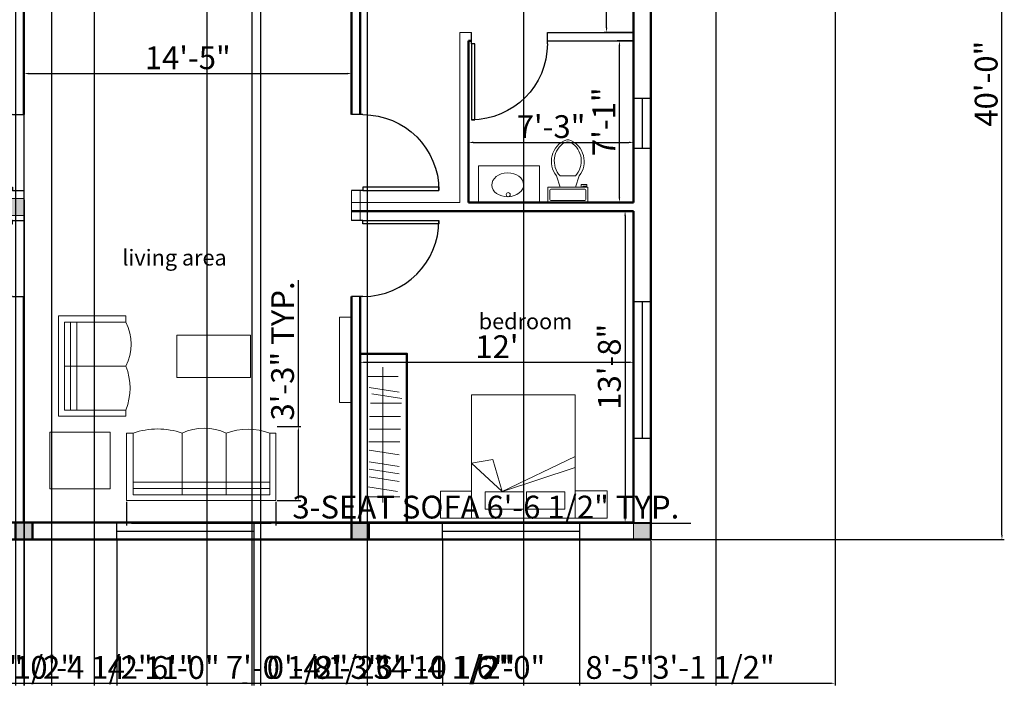
# Model space of a CAD drawing. Units: inches. Extents: x 1367 to 2309, y 1406 to 3826.
# Tile 5 of 9: x 1781 to 2300, y 2247 to 2608. Entities that reach past the tile are written whole.
import ezdxf

# ---------------------------------------------------------------- set-up
doc = ezdxf.new("R2010")
doc.units = ezdxf.units.IN
for name, color, linetype, lineweight in [('A-ANNO-DIMS', 2, 'Continuous', 18), ('A-AREA-IDEN', 3, 'Continuous', 18), ('A-DOOR', 4, 'Continuous', 25), ('A-FLOR-FIXT', 8, 'Continuous', 18), ('A-FURN', 8, 'Continuous', 18), ('A-GLAZ', 4, 'Continuous', 25), ('A-WALL', 7, 'Continuous', 50), ('A-WALL-PATT', 8, 'Continuous', 18)]:
    doc.layers.add(name, color=color, linetype=linetype, lineweight=lineweight)
doc.styles.get("Standard").update_dxf_attribs({"font": 'arial.ttf'})
doc.dimstyles.new('ISO-25', dxfattribs={"dimtxt": 12, "dimasz": 2.5, "dimexe": 1.25, "dimexo": 0.625, "dimtad": 1, "dimdec": 0, "dimlunit": 4, "dimtxsty": 'Standard', "dimcen": 2.5, "dimadec": 0, "dimazin": 0, "dimtfac": 1, "dimtdec": 0, "dimtmove": 0, "dimatfit": 3, "dimfxl": 1, "dimarcsym": 0})

# ---------------------------------------------------------------- blocks, each defined once
blk = doc.blocks.new('*U2')
for p, q in [((0, 0), (0, -6)), ((40, 0), (40, -6))]:
    blk.add_line(p, q)
blk.add_lwpolyline([(0, 0), (0, 40), (1.75, 40), (1.75, 0)], close=True)
blk.add_arc((0, 0), 40, 0, 90)
blk = doc.blocks.new('*U4')
for p, q in [((9.5, -6), (9.5, -2)), ((-10, -8.5), (-8, -8.5)), ((-10, -9.5), (-10, -8.5)), ((-7, -9.5), (-10, -9.5)), ((-8, -8.5), (-8, -8)), ((-7, -8), (-7, -9.5)), ((-4, -8), (-6, -14)), ((4, -8), (6, -14)), ((4, -14), (-4, -14))]:
    blk.add_line(p, q)
blk.add_lwpolyline([(10.5, -8), (10.5, 0), (-10.5, 0), (-10.5, -8)], close=True)
for points in [[(-9.5, -2), (-9.5, -6)], [(8.5, -1), (-8.5, -1)], [(-8.5, -7), (8.5, -7)]]:
    blk.add_lwpolyline(points)
for centre, radius, start, end in [((-8.62, -1.88), 0.884, 81.8699, 188.1301), ((8.62, -1.88), 0.884, 351.8699, 98.1301), ((-8.62, -6.12), 0.884, 171.8699, 278.1301), ((8.62, -6.12), 0.884, 261.8699, 8.1301), ((3.52, -21.58), 12.17, 141.4691, 247.9714), ((4.2, -21.82), 11.33, 136.3677, 238.9468), ((-3.52, -21.58), 12.17, 292.0284, 38.5307), ((-4.2, -21.82), 11.33, 301.053, 43.6321), ((0, -27.88), 4, 245.7318, 294.2682), ((0, -29), 4, 254.8605, 285.1395)]:
    blk.add_arc(centre, radius, start, end)
blk = doc.blocks.new('*D16')
at = {"layer": 'A-ANNO-DIMS', "color": 0, "lineweight": -2, "transparency": 16777216}
for p, q in [((2103.75, 2805.17), (2088.85, 2805.17)), ((2090.1, 2603.67), (2090.1, 2802.67)), ((2103.75, 2601.17), (2088.85, 2601.17))]:
    blk.add_line(p, q, dxfattribs=at)
at = {"layer": 'A-ANNO-DIMS', "color": 0, "lineweight": 100, "transparency": 16777216}
for points in [[(2089.68, 2802.67), (2090.51, 2802.67), (2090.1, 2805.17)], [(2089.68, 2603.67), (2090.51, 2603.67), (2090.1, 2601.17)]]:
    blk.add_solid(points, dxfattribs=at)
at = {"layer": 'Defpoints', "color": 0, "lineweight": 100, "transparency": 16777216}
for p in [(2090.1, 2805.17), (2104.37, 2805.17), (2104.37, 2601.17)]:
    blk.add_point(p, dxfattribs=at)
at = {"layer": 'A-ANNO-DIMS', "color": 0, "transparency": 16777216, "insert": (2083.45, 2703.17), "char_height": 12, "attachment_point": 5, "rotation": 90}
blk.add_mtext("17'", dxfattribs=at)
blk = doc.blocks.new('*D17')
at = {"layer": 'A-ANNO-DIMS', "color": 0, "lineweight": -2, "transparency": 16777216}
for p, q in [((2103.75, 2596.67), (2095.64, 2596.67)), ((2096.89, 2514.16), (2096.89, 2594.17)), ((2103.75, 2511.66), (2095.64, 2511.66))]:
    blk.add_line(p, q, dxfattribs=at)
at = {"layer": 'A-ANNO-DIMS', "color": 0, "lineweight": 100, "transparency": 16777216}
for points in [[(2096.47, 2594.17), (2097.3, 2594.17), (2096.89, 2596.67)], [(2096.47, 2514.16), (2097.3, 2514.16), (2096.89, 2511.66)]]:
    blk.add_solid(points, dxfattribs=at)
at = {"layer": 'Defpoints', "color": 0, "lineweight": 100, "transparency": 16777216}
for p in [(2096.89, 2596.67), (2104.37, 2596.67), (2104.37, 2511.66)]:
    blk.add_point(p, dxfattribs=at)
at = {"layer": 'A-ANNO-DIMS', "color": 0, "transparency": 16777216, "insert": (2090.24, 2554.16), "char_height": 12, "attachment_point": 5, "rotation": 90}
blk.add_mtext('7\'-1"', dxfattribs=at)
blk = doc.blocks.new('*D18')
at = {"layer": 'A-ANNO-DIMS', "color": 0, "lineweight": -2, "transparency": 16777216}
for p, q in [((2017.4, 2512.28), (2017.4, 2544.52)), ((2019.9, 2543.27), (2101.87, 2543.27)), ((2104.37, 2512.28), (2104.37, 2544.52))]:
    blk.add_line(p, q, dxfattribs=at)
at = {"layer": 'A-ANNO-DIMS', "color": 0, "lineweight": 100, "transparency": 16777216}
for points in [[(2019.9, 2543.69), (2019.9, 2542.86), (2017.4, 2543.27)], [(2101.87, 2543.69), (2101.87, 2542.86), (2104.37, 2543.27)]]:
    blk.add_solid(points, dxfattribs=at)
at = {"layer": 'Defpoints', "color": 0, "lineweight": 100, "transparency": 16777216}
for p in [(2104.37, 2543.27), (2017.4, 2511.66), (2104.37, 2511.66)]:
    blk.add_point(p, dxfattribs=at)
at = {"layer": 'A-ANNO-DIMS', "color": 0, "transparency": 16777216, "insert": (2060.89, 2550.03), "char_height": 12, "attachment_point": 5}
blk.add_mtext('7\'-3"', dxfattribs=at)
blk = doc.blocks.new('*D19')
at = {"layer": 'A-ANNO-DIMS', "color": 0, "lineweight": -2, "transparency": 16777216}
for p, q in [((1960.37, 2343.79), (1960.37, 2428.77)), ((1962.87, 2427.52), (2101.87, 2427.52)), ((2104.37, 2343.79), (2104.37, 2428.77))]:
    blk.add_line(p, q, dxfattribs=at)
at = {"layer": 'A-ANNO-DIMS', "color": 0, "lineweight": 100, "transparency": 16777216}
for points in [[(1962.87, 2427.93), (1962.87, 2427.1), (1960.37, 2427.52)], [(2101.87, 2427.93), (2101.87, 2427.1), (2104.37, 2427.52)]]:
    blk.add_solid(points, dxfattribs=at)
at = {"layer": 'Defpoints', "color": 0, "lineweight": 100, "transparency": 16777216}
for p in [(2104.37, 2427.52), (1960.37, 2343.17), (2104.37, 2343.17)]:
    blk.add_point(p, dxfattribs=at)
at = {"layer": 'A-ANNO-DIMS', "color": 0, "transparency": 16777216, "insert": (2032.37, 2434.17), "char_height": 12, "attachment_point": 5}
blk.add_mtext("12'", dxfattribs=at)
blk = doc.blocks.new('*D20')
at = {"layer": 'A-ANNO-DIMS', "color": 0, "lineweight": -2, "transparency": 16777216}
for p, q in [((2103.75, 2507.16), (2098.62, 2507.16)), ((2099.87, 2504.66), (2099.87, 2345.67)), ((2103.75, 2343.17), (2098.62, 2343.17))]:
    blk.add_line(p, q, dxfattribs=at)
at = {"layer": 'A-ANNO-DIMS', "color": 0, "lineweight": 100, "transparency": 16777216}
for points in [[(2099.46, 2504.66), (2100.29, 2504.66), (2099.87, 2507.16)], [(2099.46, 2345.67), (2100.29, 2345.67), (2099.87, 2343.17)]]:
    blk.add_solid(points, dxfattribs=at)
at = {"layer": 'Defpoints', "color": 0, "lineweight": 100, "transparency": 16777216}
for p in [(2104.37, 2507.16), (2099.87, 2343.17), (2104.37, 2343.17)]:
    blk.add_point(p, dxfattribs=at)
at = {"layer": 'A-ANNO-DIMS', "color": 0, "transparency": 16777216, "insert": (2093.12, 2425.16), "char_height": 12, "attachment_point": 5, "rotation": 90}
blk.add_mtext('13\'-8"', dxfattribs=at)
blk = doc.blocks.new('*D37')
at = {"layer": 'A-ANNO-DIMS', "color": 0, "lineweight": -2, "transparency": 16777216}
for p, q in [((1783.37, 2558.52), (1783.37, 2580.77)), ((1785.87, 2579.52), (1953.37, 2579.52)), ((1955.87, 2558.52), (1955.87, 2580.77))]:
    blk.add_line(p, q, dxfattribs=at)
at = {"layer": 'A-ANNO-DIMS', "color": 0, "lineweight": 100, "transparency": 16777216}
for points in [[(1785.87, 2579.94), (1785.87, 2579.1), (1783.37, 2579.52)], [(1953.37, 2579.94), (1953.37, 2579.1), (1955.87, 2579.52)]]:
    blk.add_solid(points, dxfattribs=at)
at = {"layer": 'Defpoints', "color": 0, "lineweight": 100, "transparency": 16777216}
for p in [(1955.87, 2579.52), (1783.37, 2557.89), (1955.87, 2557.89)]:
    blk.add_point(p, dxfattribs=at)
at = {"layer": 'A-ANNO-DIMS', "color": 0, "transparency": 16777216, "insert": (1869.62, 2586.27), "char_height": 12, "attachment_point": 5}
blk.add_mtext('14\'-5"', dxfattribs=at)
blk = doc.blocks.new('SOFA-3')
for p, q in [((3.39, 35.52), (0, 35.52)), ((0, 35.52), (0, 0)), ((29.28, 35.52), (29.28, 3.13)), ((52.37, 35.52), (52.37, 3.13)), ((75.45, 35.52), (78.61, 35.52)), ((78.61, 0), (78.61, 35.52)), ((0, 0), (78.61, 0))]:
    blk.add_line(p, q)
blk.add_lwpolyline([(3.39, 35.52), (3.39, 3.13), (75.45, 3.13), (75.45, 35.52)])
for centre, radius, start, end in [((16.33, -1.36), 39.09, 70.661, 109.339), ((40.82, 12.11), 26.1, 63.7496, 116.2504), ((63.91, 5.49), 32.17, 68.9718, 111.0282)]:
    blk.add_arc(centre, radius, start, end)
blk = doc.blocks.new('ARMCHAIR')
for p, q in [((0, 52.73), (0, 0)), ((35.52, 52.73), (0, 52.73)), ((35.52, 49.34), (35.52, 52.73)), ((35.52, 49.34), (3.13, 49.34)), ((35.52, 26.25), (3.13, 26.25)), ((35.52, 3.16), (35.52, 0)), ((0, 0), (35.52, 0))]:
    blk.add_line(p, q)
blk.add_lwpolyline([(3.13, 49.34), (3.13, 3.16), (35.52, 3.16)])
for centre, radius, start, end in [((12.11, 37.79), 26.1, 333.7496, 26.2504), ((5.49, 14.7), 32.17, 338.9718, 21.0282)]:
    blk.add_arc(centre, radius, start, end)
blk = doc.blocks.new('*D51')
at = {"layer": 'A-ANNO-DIMS', "color": 0, "lineweight": -2, "transparency": 16777216}
for p, q in [((1837.44, 2354.05), (1837.44, 2341.63)), ((1916.05, 2354.05), (1916.05, 2341.63)), ((1839.94, 2342.88), (1913.55, 2342.88)), ((1916.05, 2342.88), (2134.55, 2342.88))]:
    blk.add_line(p, q, dxfattribs=at)
at = {"layer": 'A-ANNO-DIMS', "color": 0, "lineweight": 100, "transparency": 16777216}
for points in [[(1839.94, 2343.3), (1839.94, 2342.47), (1837.44, 2342.88)], [(1913.55, 2343.3), (1913.55, 2342.47), (1916.05, 2342.88)]]:
    blk.add_solid(points, dxfattribs=at)
at = {"layer": 'Defpoints', "color": 0, "lineweight": 100, "transparency": 16777216}
for p in [(1837.44, 2354.68), (1916.05, 2354.68), (1916.05, 2342.88)]:
    blk.add_point(p, dxfattribs=at)
at = {"layer": 'A-ANNO-DIMS', "color": 0, "transparency": 16777216, "insert": (2026.55, 2349.72), "char_height": 12, "attachment_point": 5}
blk.add_mtext('3-SEAT SOFA 6\'-6 1/2" TYP.', dxfattribs=at)
blk = doc.blocks.new('*D52')
at = {"layer": 'A-ANNO-DIMS', "color": 0, "lineweight": -2, "transparency": 16777216}
for p, q in [((1927.84, 2393.78), (1927.84, 2470.67)), ((1916.67, 2393.78), (1929.09, 2393.78)), ((1927.84, 2357.18), (1927.84, 2391.28)), ((1916.67, 2354.68), (1929.09, 2354.68))]:
    blk.add_line(p, q, dxfattribs=at)
at = {"layer": 'A-ANNO-DIMS', "color": 0, "lineweight": 100, "transparency": 16777216}
for points in [[(1927.43, 2391.28), (1928.26, 2391.28), (1927.84, 2393.78)], [(1927.43, 2357.18), (1928.26, 2357.18), (1927.84, 2354.68)]]:
    blk.add_solid(points, dxfattribs=at)
at = {"layer": 'Defpoints', "color": 0, "lineweight": 100, "transparency": 16777216}
for p in [(1916.05, 2393.78), (1927.84, 2393.78), (1916.05, 2354.68)]:
    blk.add_point(p, dxfattribs=at)
at = {"layer": 'A-ANNO-DIMS', "color": 0, "transparency": 16777216, "insert": (1921.09, 2433.48), "char_height": 12, "attachment_point": 5, "rotation": 90}
blk.add_mtext('3\'-3" TYP.', dxfattribs=at)
blk = doc.blocks.new('*D89')
at = {"layer": 'A-ANNO-DIMS', "color": 0, "lineweight": -2, "transparency": 16777216}
for p, q in [((2114.03, 2814.17), (2299.51, 2814.17)), ((2298.26, 2336.67), (2298.26, 2811.67)), ((2114, 2334.17), (2299.51, 2334.17))]:
    blk.add_line(p, q, dxfattribs=at)
at = {"layer": 'A-ANNO-DIMS', "color": 0, "lineweight": 100, "transparency": 16777216}
for points in [[(2297.84, 2811.67), (2298.67, 2811.67), (2298.26, 2814.17)], [(2297.84, 2336.67), (2298.67, 2336.67), (2298.26, 2334.17)]]:
    blk.add_solid(points, dxfattribs=at)
at = {"layer": 'Defpoints', "color": 0, "lineweight": 100, "transparency": 16777216}
for p in [(2113.4, 2814.17), (2298.26, 2814.17), (2113.37, 2334.17)]:
    blk.add_point(p, dxfattribs=at)
at = {"layer": 'A-ANNO-DIMS', "color": 0, "transparency": 16777216, "insert": (2291.51, 2574.17), "char_height": 12, "attachment_point": 5, "rotation": 90}
blk.add_mtext('40\'-0"', dxfattribs=at)
blk = doc.blocks.new('*D97')
at = {"layer": 'A-ANNO-DIMS', "color": 0, "lineweight": -2, "transparency": 16777216}
for p, q in [((1723.94, 2333.54), (1723.94, 2257.28)), ((1832.26, 2333.54), (1832.26, 2257.28)), ((1726.44, 2258.53), (1829.76, 2258.53))]:
    blk.add_line(p, q, dxfattribs=at)
at = {"layer": 'A-ANNO-DIMS', "color": 0, "lineweight": 100, "transparency": 16777216}
for points in [[(1726.44, 2258.94), (1726.44, 2258.11), (1723.94, 2258.53)], [(1829.76, 2258.94), (1829.76, 2258.11), (1832.26, 2258.53)]]:
    blk.add_solid(points, dxfattribs=at)
at = {"layer": 'Defpoints', "color": 0, "lineweight": 100, "transparency": 16777216}
for p in [(1723.94, 2334.17), (1832.26, 2334.17), (1832.26, 2258.53)]:
    blk.add_point(p, dxfattribs=at)
at = {"layer": 'A-ANNO-DIMS', "color": 0, "transparency": 16777216, "insert": (1778.1, 2265.35), "char_height": 12, "attachment_point": 5}
blk.add_mtext('9\'-0 1/2"', dxfattribs=at)
blk = doc.blocks.new('*D98')
at = {"layer": 'A-ANNO-DIMS', "color": 0, "lineweight": -2, "transparency": 16777216}
for p, q in [((1832.26, 2333.54), (1832.26, 2257.28)), ((1904.42, 2333.54), (1904.42, 2257.28)), ((1834.76, 2258.53), (1901.92, 2258.53))]:
    blk.add_line(p, q, dxfattribs=at)
at = {"layer": 'A-ANNO-DIMS', "color": 0, "lineweight": 100, "transparency": 16777216}
for points in [[(1834.76, 2258.94), (1834.76, 2258.11), (1832.26, 2258.53)], [(1901.92, 2258.94), (1901.92, 2258.11), (1904.42, 2258.53)]]:
    blk.add_solid(points, dxfattribs=at)
at = {"layer": 'Defpoints', "color": 0, "lineweight": 100, "transparency": 16777216}
for p in [(1832.26, 2334.17), (1904.42, 2334.17), (1904.42, 2258.53)]:
    blk.add_point(p, dxfattribs=at)
at = {"layer": 'A-ANNO-DIMS', "color": 0, "transparency": 16777216, "insert": (1868.34, 2265.28), "char_height": 12, "attachment_point": 5}
blk.add_mtext('6\'-0"', dxfattribs=at)
blk = doc.blocks.new('*D99')
at = {"layer": 'A-ANNO-DIMS', "color": 0, "lineweight": -2, "transparency": 16777216}
for p, q in [((1904.42, 2333.54), (1904.42, 2257.28)), ((2003.66, 2333.54), (2003.66, 2257.28)), ((1906.92, 2258.53), (2001.16, 2258.53))]:
    blk.add_line(p, q, dxfattribs=at)
at = {"layer": 'A-ANNO-DIMS', "color": 0, "lineweight": 100, "transparency": 16777216}
for points in [[(1906.92, 2258.94), (1906.92, 2258.11), (1904.42, 2258.53)], [(2001.16, 2258.94), (2001.16, 2258.11), (2003.66, 2258.53)]]:
    blk.add_solid(points, dxfattribs=at)
at = {"layer": 'Defpoints', "color": 0, "lineweight": 100, "transparency": 16777216}
for p in [(1904.42, 2334.17), (2003.66, 2334.17), (2003.66, 2258.53)]:
    blk.add_point(p, dxfattribs=at)
at = {"layer": 'A-ANNO-DIMS', "color": 0, "transparency": 16777216, "insert": (1954.04, 2265.28), "char_height": 12, "attachment_point": 5}
blk.add_mtext('8\'-3"', dxfattribs=at)
blk = doc.blocks.new('*D100')
at = {"layer": 'A-ANNO-DIMS', "color": 0, "lineweight": -2, "transparency": 16777216}
for p, q in [((2003.66, 2333.54), (2003.66, 2257.28)), ((2075.83, 2333.54), (2075.83, 2257.28)), ((2006.16, 2258.53), (2073.33, 2258.53))]:
    blk.add_line(p, q, dxfattribs=at)
at = {"layer": 'A-ANNO-DIMS', "color": 0, "lineweight": 100, "transparency": 16777216}
for points in [[(2006.16, 2258.94), (2006.16, 2258.11), (2003.66, 2258.53)], [(2073.33, 2258.94), (2073.33, 2258.11), (2075.83, 2258.53)]]:
    blk.add_solid(points, dxfattribs=at)
at = {"layer": 'Defpoints', "color": 0, "lineweight": 100, "transparency": 16777216}
for p in [(2003.66, 2334.17), (2075.83, 2334.17), (2075.83, 2258.53)]:
    blk.add_point(p, dxfattribs=at)
at = {"layer": 'A-ANNO-DIMS', "color": 0, "transparency": 16777216, "insert": (2039.74, 2265.28), "char_height": 12, "attachment_point": 5}
blk.add_mtext('6\'-0"', dxfattribs=at)
blk = doc.blocks.new('*D101')
at = {"layer": 'A-ANNO-DIMS', "color": 0, "lineweight": -2, "transparency": 16777216}
for p, q in [((2075.83, 2333.54), (2075.83, 2257.28)), ((2113.37, 2333.54), (2113.37, 2257.28)), ((2078.33, 2258.53), (2110.87, 2258.53)), ((2113.37, 2258.53), (2176.97, 2258.53))]:
    blk.add_line(p, q, dxfattribs=at)
at = {"layer": 'A-ANNO-DIMS', "color": 0, "lineweight": 100, "transparency": 16777216}
for points in [[(2078.33, 2258.94), (2078.33, 2258.11), (2075.83, 2258.53)], [(2110.87, 2258.94), (2110.87, 2258.11), (2113.37, 2258.53)]]:
    blk.add_solid(points, dxfattribs=at)
at = {"layer": 'Defpoints', "color": 0, "lineweight": 100, "transparency": 16777216}
for p in [(2075.83, 2334.17), (2113.37, 2334.17), (2113.37, 2258.53)]:
    blk.add_point(p, dxfattribs=at)
at = {"layer": 'A-ANNO-DIMS', "color": 0, "transparency": 16777216, "insert": (2146.42, 2265.36), "char_height": 12, "attachment_point": 5}
blk.add_mtext('3\'-1 1/2"', dxfattribs=at)
blk = doc.blocks.new('*D102')
at = {"layer": 'A-ANNO-DIMS', "color": 0, "lineweight": -2, "transparency": 16777216}
for p, q in [((1778.87, 2804.54), (1778.87, 2257.28)), ((1783.37, 2804.54), (1783.37, 2257.28)), ((1776.37, 2258.53), (1773.87, 2258.53)), ((1778.87, 2258.53), (1783.37, 2258.53)), ((1785.87, 2258.53), (1849.48, 2258.53))]:
    blk.add_line(p, q, dxfattribs=at)
at = {"layer": 'A-ANNO-DIMS', "color": 0, "lineweight": 100, "transparency": 16777216}
for points in [[(1776.37, 2258.94), (1776.37, 2258.11), (1778.87, 2258.53)], [(1785.87, 2258.94), (1785.87, 2258.11), (1783.37, 2258.53)]]:
    blk.add_solid(points, dxfattribs=at)
at = {"layer": 'Defpoints', "color": 0, "lineweight": 100, "transparency": 16777216}
for p in [(1778.87, 2805.17), (1783.37, 2805.17), (1783.37, 2258.53)]:
    blk.add_point(p, dxfattribs=at)
at = {"layer": 'A-ANNO-DIMS', "color": 0, "transparency": 16777216, "insert": (1818.93, 2265.35), "char_height": 12, "attachment_point": 5}
blk.add_mtext('0\'-4 1/2"', dxfattribs=at)
blk = doc.blocks.new('*D113')
at = {"layer": 'A-ANNO-DIMS', "color": 0, "lineweight": -2, "transparency": 16777216}
for p, q in [((1797.9, 3128.9), (1797.9, 2257.28)), ((2210.4, 3128.9), (2210.4, 2257.28)), ((1800.4, 2258.53), (2207.9, 2258.53))]:
    blk.add_line(p, q, dxfattribs=at)
at = {"layer": 'A-ANNO-DIMS', "color": 0, "lineweight": 100, "transparency": 16777216}
for points in [[(1800.4, 2258.94), (1800.4, 2258.11), (1797.9, 2258.53)], [(2207.9, 2258.94), (2207.9, 2258.11), (2210.4, 2258.53)]]:
    blk.add_solid(points, dxfattribs=at)
at = {"layer": 'Defpoints', "color": 0, "lineweight": 100, "transparency": 16777216}
for p in [(1797.9, 3129.52), (2210.4, 3129.52), (2210.4, 2258.53)]:
    blk.add_point(p, dxfattribs=at)
at = {"layer": 'A-ANNO-DIMS', "color": 0, "transparency": 16777216, "insert": (2004.15, 2265.36), "char_height": 12, "attachment_point": 5}
blk.add_mtext('34\'-4 1/2"', dxfattribs=at)
blk = doc.blocks.new('*D114')
at = {"layer": 'A-ANNO-DIMS', "color": 0, "lineweight": -2, "transparency": 16777216}
for p, q in [((1820.42, 3150.44), (1820.42, 2257.28)), ((1879.66, 3150.44), (1879.66, 2257.28)), ((1822.92, 2258.53), (1877.16, 2258.53))]:
    blk.add_line(p, q, dxfattribs=at)
at = {"layer": 'A-ANNO-DIMS', "color": 0, "lineweight": 100, "transparency": 16777216}
for points in [[(1822.92, 2258.94), (1822.92, 2258.11), (1820.42, 2258.53)], [(1877.16, 2258.94), (1877.16, 2258.11), (1879.66, 2258.53)]]:
    blk.add_solid(points, dxfattribs=at)
at = {"layer": 'Defpoints', "color": 0, "lineweight": 100, "transparency": 16777216}
for p in [(1820.42, 3151.06), (1879.66, 3151.06), (1879.66, 2258.53)]:
    blk.add_point(p, dxfattribs=at)
at = {"layer": 'A-ANNO-DIMS', "color": 0, "transparency": 16777216, "insert": (1850.04, 2265.17), "char_height": 12, "attachment_point": 5}
blk.add_mtext('4\'-11"', dxfattribs=at)
blk = doc.blocks.new('*D115')
at = {"layer": 'A-ANNO-DIMS', "color": 0, "lineweight": -2, "transparency": 16777216}
for p, q in [((1879.66, 3150.44), (1879.66, 2257.28)), ((1964.13, 3150.44), (1964.13, 2257.28)), ((1882.16, 2258.53), (1961.63, 2258.53))]:
    blk.add_line(p, q, dxfattribs=at)
at = {"layer": 'A-ANNO-DIMS', "color": 0, "lineweight": 100, "transparency": 16777216}
for points in [[(1882.16, 2258.94), (1882.16, 2258.11), (1879.66, 2258.53)], [(1961.63, 2258.94), (1961.63, 2258.11), (1964.13, 2258.53)]]:
    blk.add_solid(points, dxfattribs=at)
at = {"layer": 'Defpoints', "color": 0, "lineweight": 100, "transparency": 16777216}
for p in [(1879.66, 3151.06), (1964.13, 3151.06), (1964.13, 2258.53)]:
    blk.add_point(p, dxfattribs=at)
at = {"layer": 'A-ANNO-DIMS', "color": 0, "transparency": 16777216, "insert": (1921.89, 2265.35), "char_height": 12, "attachment_point": 5}
blk.add_mtext('7\'-0 1/2"', dxfattribs=at)
blk = doc.blocks.new('*D116')
at = {"layer": 'A-ANNO-DIMS', "color": 0, "lineweight": -2, "transparency": 16777216}
for p, q in [((1964.13, 3150.44), (1964.13, 2257.28)), ((2046.46, 3150.44), (2046.46, 2257.28)), ((1966.63, 2258.53), (2043.96, 2258.53))]:
    blk.add_line(p, q, dxfattribs=at)
at = {"layer": 'A-ANNO-DIMS', "color": 0, "lineweight": 100, "transparency": 16777216}
for points in [[(1966.63, 2258.94), (1966.63, 2258.11), (1964.13, 2258.53)], [(2043.96, 2258.94), (2043.96, 2258.11), (2046.46, 2258.53)]]:
    blk.add_solid(points, dxfattribs=at)
at = {"layer": 'Defpoints', "color": 0, "lineweight": 100, "transparency": 16777216}
for p in [(1964.13, 3151.06), (2046.46, 3151.06), (2046.46, 2258.53)]:
    blk.add_point(p, dxfattribs=at)
at = {"layer": 'A-ANNO-DIMS', "color": 0, "transparency": 16777216, "insert": (2005.29, 2265.35), "char_height": 12, "attachment_point": 5}
blk.add_mtext('6\'-10 1/2"', dxfattribs=at)
blk = doc.blocks.new('*D117')
at = {"layer": 'A-ANNO-DIMS', "color": 0, "lineweight": -2, "transparency": 16777216}
for p, q in [((2046.46, 3150.44), (2046.46, 2257.28)), ((2147.64, 3150.44), (2147.64, 2257.28)), ((2048.96, 2258.53), (2145.14, 2258.53))]:
    blk.add_line(p, q, dxfattribs=at)
at = {"layer": 'A-ANNO-DIMS', "color": 0, "lineweight": 100, "transparency": 16777216}
for points in [[(2048.96, 2258.94), (2048.96, 2258.11), (2046.46, 2258.53)], [(2145.14, 2258.94), (2145.14, 2258.11), (2147.64, 2258.53)]]:
    blk.add_solid(points, dxfattribs=at)
at = {"layer": 'Defpoints', "color": 0, "lineweight": 100, "transparency": 16777216}
for p in [(2046.46, 3151.06), (2147.64, 3151.06), (2147.64, 2258.53)]:
    blk.add_point(p, dxfattribs=at)
at = {"layer": 'A-ANNO-DIMS', "color": 0, "transparency": 16777216, "insert": (2097.05, 2265.28), "char_height": 12, "attachment_point": 5}
blk.add_mtext('8\'-5"', dxfattribs=at)
blk = doc.blocks.new('*D135')
at = {"layer": 'A-ANNO-DIMS', "color": 0, "lineweight": -2, "transparency": 16777216}
for p, q in [((1903.37, 2636.69), (1903.37, 2257.28)), ((1907.87, 2632.19), (1907.87, 2257.28)), ((1900.87, 2258.53), (1898.37, 2258.53)), ((1903.37, 2258.53), (1907.87, 2258.53)), ((1910.37, 2258.53), (1973.98, 2258.53))]:
    blk.add_line(p, q, dxfattribs=at)
at = {"layer": 'A-ANNO-DIMS', "color": 0, "lineweight": 100, "transparency": 16777216}
for points in [[(1900.87, 2258.94), (1900.87, 2258.11), (1903.37, 2258.53)], [(1910.37, 2258.94), (1910.37, 2258.11), (1907.87, 2258.53)]]:
    blk.add_solid(points, dxfattribs=at)
at = {"layer": 'Defpoints', "color": 0, "lineweight": 100, "transparency": 16777216}
for p in [(1903.37, 2637.31), (1907.87, 2632.81), (1907.87, 2258.53)]:
    blk.add_point(p, dxfattribs=at)
at = {"layer": 'A-ANNO-DIMS', "color": 0, "transparency": 16777216, "insert": (1943.43, 2265.35), "char_height": 12, "attachment_point": 5}
blk.add_mtext('0\'-4 1/2"', dxfattribs=at)
blk = doc.blocks.new('*D138')
at = {"layer": 'A-ANNO-DIMS', "color": 0, "lineweight": -2, "transparency": 16777216}
for p, q in [((1737.37, 2517.27), (1737.37, 2257.28)), ((1783.44, 2513.11), (1783.44, 2257.28)), ((1739.87, 2258.53), (1780.94, 2258.53))]:
    blk.add_line(p, q, dxfattribs=at)
at = {"layer": 'A-ANNO-DIMS', "color": 0, "lineweight": 100, "transparency": 16777216}
for points in [[(1739.87, 2258.94), (1739.87, 2258.11), (1737.37, 2258.53)], [(1780.94, 2258.94), (1780.94, 2258.11), (1783.44, 2258.53)]]:
    blk.add_solid(points, dxfattribs=at)
at = {"layer": 'Defpoints', "color": 0, "lineweight": 100, "transparency": 16777216}
for p in [(1737.37, 2517.89), (1783.44, 2513.73), (1783.44, 2258.53)]:
    blk.add_point(p, dxfattribs=at)
at = {"layer": 'A-ANNO-DIMS', "color": 0, "transparency": 16777216, "insert": (1760.4, 2265.28), "char_height": 12, "attachment_point": 5}
blk.add_mtext('3\'-10"', dxfattribs=at)

msp = doc.modelspace()

# ---------------------------------------------------------------- hatches: boundary and pattern name
at = {"layer": 'A-WALL-PATT'}
h = msp.add_hatch(color=256, dxfattribs=at)
h.dxf.hatch_style = 1
h.paths.add_polyline_path([(1513.37, 2983.62), (1504.37, 2983.62), (1504.37, 2974.62), (1513.37, 2974.62)])
h.paths.add_polyline_path([(1759.42, 2983.62), (1749.82, 2983.62), (1749.82, 2974.62), (1759.42, 2974.62)])
h.paths.add_polyline_path([(1513.37, 3283.62), (1504.37, 3283.62), (1504.37, 3274.62), (1513.37, 3274.62)])
h.paths.add_polyline_path([(1759.42, 3283.62), (1750.75, 3283.62), (1750.75, 3274.62), (1759.42, 3274.62)])
h.paths.add_polyline_path([(2113.4, 2983.62), (2104.4, 2983.62), (2104.4, 2974.62), (2113.4, 2974.62)])
h.paths.add_polyline_path([(1787.87, 2343.17), (1778.87, 2343.17), (1778.87, 2334.17), (1787.87, 2334.17)])
h.paths.add_polyline_path([(1964.87, 2343.17), (1960.37, 2343.17), (1955.87, 2343.17), (1955.87, 2334.17), (1964.87, 2334.17)])
h.paths.add_polyline_path([(2113.37, 2343.17), (2104.37, 2343.17), (2104.37, 2334.17), (2113.37, 2334.17)])
h.paths.add_polyline_path([(1783.37, 2513.73), (1774.44, 2513.73), (1774.44, 2504.73), (1783.37, 2504.73)])
h.paths.add_polyline_path([(1787.54, 2814.17), (1778.54, 2814.17), (1778.54, 2805.17), (1787.54, 2805.17)])
h.paths.add_polyline_path([(1964.87, 2814.17), (1955.87, 2814.17), (1955.87, 2805.17), (1964.87, 2805.17)])
h.paths.add_polyline_path([(2113.37, 2814.17), (2104.4, 2814.17), (2104.4, 2805.17), (2113.37, 2805.17)])
h.paths.add_polyline_path([(1522.37, 2814.17), (1513.37, 2814.17), (1513.37, 2805.17), (1522.37, 2805.17)])
h.paths.add_polyline_path([(2019.97, 2440.35), (2070.2, 2440.35), (2070.2, 2457.56), (2019.97, 2457.56)], flags=9)
h.paths.add_polyline_path([(1670.17, 2422.1), (1711.32, 2422.1), (1711.32, 2439.31), (1670.17, 2439.31)], flags=9)
h.paths.add_polyline_path([(1917.64, 2783.38), (1946.46, 2783.38), (1946.46, 2800.59), (1917.64, 2800.59)], flags=9)
h.paths.add_polyline_path([(1526.17, 2423.16), (1570.57, 2423.16), (1570.57, 2440.37), (1526.17, 2440.37)], flags=9)
h.paths.add_polyline_path([(2013.98, 2676.57), (2064.21, 2676.57), (2064.21, 2693.79), (2013.98, 2693.79)], flags=9)
h.paths.add_polyline_path([(1738.47, 2785.04), (1767.29, 2785.04), (1767.29, 2802.25), (1738.47, 2802.25)], flags=9)
h.paths.add_polyline_path([(1832.32, 2473.89), (1889.69, 2473.89), (1889.69, 2491.1), (1832.32, 2491.1)], flags=9)
h.paths.add_polyline_path([(1821.9, 2712.75), (1863.05, 2712.75), (1863.05, 2729.96), (1821.9, 2729.96)], flags=9)
h.paths.add_polyline_path([(1595.64, 2683.62), (1684.77, 2683.62), (1684.77, 2700.83), (1595.64, 2700.83)], flags=9)

# ---------------------------------------------------------------- linework, layer by layer
at = {"layer": 'A-FURN'}
for p, q in [((2012.9, 2601.17), (2018.94, 2601.17)), ((2012.9, 2596.67), (2012.9, 2601.17)), ((2012.9, 2597.06), (2012.9, 2511.66)), ((2022.62, 2511.66), (2022.62, 2531.01)), ((1783.37, 2517.89), (1783.37, 2502.15)), ((1955.87, 2517.89), (1955.87, 2502.15)), ((1960.37, 2517.89), (1960.37, 2502.15)), ((1960.37, 2517.89), (1960.37, 2511.66)), ((2012.9, 2511.66), (1955.87, 2511.66)), ((1960.37, 2507.16), (1960.37, 2502.15)), ((1807.88, 2448.57), (1807.88, 2402.39)), ((1811.23, 2448.57), (1811.23, 2402.39)), ((1972.25, 2353.72), (1972.25, 2424.98)), ((1980.4, 2420.01), (1964.09, 2420.01)), ((1980.87, 2411.85), (1965.2, 2414.3)), ((1982.28, 2408.39), (1966.61, 2410.84)), ((1982.15, 2405.93), (1965.83, 2405.93)), ((1981.68, 2399.01), (1965.37, 2399.01)), ((1981.68, 2392.32), (1965.37, 2392.32)), ((1981.18, 2385.63), (1964.86, 2385.63)), ((1980.87, 2378.74), (1965.2, 2381.19)), ((1980.87, 2372.6), (1965.2, 2375.06)), ((2019.02, 2374.34), (2030.23, 2376.29)), ((2035.09, 2359.48), (2019.02, 2374.34)), ((2030.23, 2376.29), (2035.09, 2359.48)), ((2034.75, 2359.32), (2073.57, 2377.96)), ((1980.87, 2368.72), (1965.2, 2371.18)), ((2034.75, 2359.32), (2073.57, 2372.04)), ((1840.82, 2364.35), (1912.89, 2364.35)), ((1980.87, 2364.84), (1965.2, 2367.3)), ((1840.82, 2361.01), (1912.89, 2361.01)), ((1980.02, 2359.52), (1964.36, 2361.97)), ((1981.18, 2356.63), (1964.86, 2356.63)), ((1967.61, 2356.63), (1981.18, 2356.63))]:
    msp.add_line(p, q, dxfattribs=at)
for points in [[(2022.62, 2531.01), (2022.62, 2511.66), (2054.8, 2511.66), (2054.8, 2531.01)], [(1774.44, 2513.73), (1783.44, 2513.73), (1783.44, 2504.73), (1774.44, 2504.73)], [(1955.87, 2451.25), (1949.51, 2451.25), (1949.51, 2406.28), (1955.87, 2406.28)], [(1863.92, 2441.81), (1902.73, 2441.81), (1902.73, 2419.48), (1863.92, 2419.48)], [(2073.57, 2345.49), (2019.02, 2345.49), (2019.02, 2410.42), (2073.57, 2410.42)], [(1796.98, 2360.83), (1828.7, 2360.83), (1828.7, 2390.66), (1796.98, 2390.66)], [(2019.02, 2345.49), (2002.75, 2345.49), (2002.75, 2359.75), (2019.02, 2359.75)], [(2046.33, 2350.12), (2026.14, 2350.12), (2026.14, 2359.32), (2046.33, 2359.32)], [(2068.21, 2350.12), (2048.01, 2350.12), (2048.01, 2359.32), (2068.21, 2359.32)], [(2073.57, 2345.49), (2090.39, 2345.49), (2090.39, 2359.89), (2073.57, 2359.89)], [(2104.37, 2343.17), (2113.37, 2343.17), (2113.37, 2334.17), (2104.37, 2334.17)]]:
    msp.add_lwpolyline(points, close=True, dxfattribs=at)
msp.add_circle((2038.32, 2515.76), 1.06, dxfattribs=at)
msp.add_ellipse((2038.06, 2520.97), major_axis=(8.38, 0.17), ratio=0.747916, dxfattribs=at)
at = {"layer": 'A-GLAZ'}
for p, q in [((2058.94, 2601.17), (2104.37, 2601.17)), ((2058.94, 2596.67), (2104.37, 2596.67)), ((2108.87, 2566.33), (2108.87, 2540.26)), ((2108.87, 2459.57), (2108.87, 2387.4)), ((1832.26, 2338.67), (1904.42, 2338.67)), ((2003.66, 2338.67), (2075.83, 2338.67))]:
    msp.add_line(p, q, dxfattribs=at)
for points in [[(2104.37, 2566.33), (2104.37, 2540.26), (2113.37, 2540.26), (2113.37, 2566.33)], [(2113.37, 2459.57), (2113.37, 2387.4), (2104.37, 2387.4), (2104.37, 2459.57)], [(1832.26, 2343.17), (1904.42, 2343.17), (1904.42, 2334.17), (1832.26, 2334.17)], [(2003.66, 2343.17), (2075.83, 2343.17), (2075.83, 2334.17), (2003.66, 2334.17)]]:
    msp.add_lwpolyline(points, close=True, dxfattribs=at)
at = {"layer": 'A-WALL'}
for p, q in [((1955.87, 2805.17), (1955.87, 2596.67)), ((1960.37, 2805.17), (1960.37, 2601.17)), ((1783.37, 2601.17), (1783.37, 2632.81)), ((1783.37, 2601.17), (1783.37, 2557.89)), ((1960.37, 2601.17), (1960.37, 2557.89)), ((1955.87, 2596.67), (1955.87, 2557.89)), ((1960.37, 2596.67), (1960.37, 2557.89)), ((2017.4, 2596.67), (2017.4, 2511.66)), ((2017.4, 2596.67), (2018.94, 2596.67)), ((2101.46, 2511.66), (2017.4, 2511.66)), ((2101.46, 2511.66), (2104.37, 2511.66)), ((2012.9, 2507.16), (1955.87, 2507.16)), ((2101.46, 2507.16), (2012.9, 2507.16)), ((2101.46, 2507.16), (2104.37, 2507.16)), ((1783.37, 2462.15), (1783.37, 2343.17)), ((1955.87, 2462.15), (1955.87, 2343.17)), ((1960.37, 2462.15), (1960.37, 2343.17))]:
    msp.add_line(p, q, dxfattribs=at)
for points in [[(1513.37, 2334.17), (2113.37, 2334.17), (2113.37, 2814.17), (1513.37, 2814.17)], [(1960.37, 2343.17), (1985.01, 2343.17), (1985.01, 2432.02), (1960.37, 2432.02)], [(1778.87, 2343.17), (1787.87, 2343.17), (1787.87, 2334.17), (1778.87, 2334.17)], [(1955.87, 2343.17), (1964.87, 2343.17), (1964.87, 2334.17), (1955.87, 2334.17)]]:
    msp.add_lwpolyline(points, close=True, dxfattribs=at)
for points in [[(2104.37, 2511.66), (2104.37, 2805.17), (1522.37, 2805.17), (1522.37, 2507.16)], [(1960.37, 2343.17), (2104.37, 2343.17), (2104.37, 2507.16)], [(1606.37, 2343.17), (1955.87, 2343.17)]]:
    msp.add_lwpolyline(points, dxfattribs=at)

# ---------------------------------------------------------------- block references
at = {"layer": 'A-DOOR', "xscale": -1}
for p, rotation in [((2018.94, 2595.17), 180), ((1961.87, 2517.89), 270), ((1777.37, 2502.15), 90)]:
    msp.add_blockref('*U2', p, dxfattribs=dict(at, rotation=rotation))
at = {"layer": 'A-DOOR'}
for p, rotation in [((1777.37, 2517.89), 90), ((1961.87, 2502.15), 270)]:
    msp.add_blockref('*U2', p, dxfattribs=dict(at, rotation=rotation))
at = {"layer": 'A-FLOR-FIXT', "rotation": 180}
msp.add_blockref('*U4', (2069.69, 2511.66), dxfattribs=at)
at = {"layer": 'A-FURN'}
for name, p in [('ARMCHAIR', (1801.55, 2399.23)), ('SOFA-3', (1837.44, 2354.68))]:
    msp.add_blockref(name, p, dxfattribs=at)

# ---------------------------------------------------------------- texts
at = {"layer": 'A-AREA-IDEN', "attachment_point": 1}
for s, insert, char_height in [('living area', (1835.16, 2486.8), 8.3529), ('bedroom', (2022.82, 2453.27), 8.353)]:
    msp.add_mtext_dynamic_manual_height_columns(s, width=204.251, gutter_width=41.76, heights=[0], dxfattribs=dict(at, insert=insert, char_height=char_height))

# ---------------------------------------------------------------- dimensions: what is measured, and where the dimension line sits
at = {"layer": 'A-ANNO-DIMS'}
for base, p1, p2, override, picture, middle in [((1879.66, 2258.53), (1820.42, 3151.06), (1879.66, 3151.06), {"dimdec": 1, "dimlfac": 1, "dimrnd": 0, "dimzin": 1, "dimdsep": 46, "dimlunit": 4, "dimfrac": 2}, '*D114', (1850.04, 2265.17)), ((1964.13, 2258.53), (1879.66, 3151.06), (1964.13, 3151.06), {"dimdec": 1, "dimlfac": 1, "dimrnd": 0, "dimzin": 1, "dimdsep": 46, "dimlunit": 4, "dimfrac": 2}, '*D115', (1921.89, 2265.35)), ((2046.46, 2258.53), (1964.13, 3151.06), (2046.46, 3151.06), {"dimdec": 1, "dimlfac": 1, "dimrnd": 0, "dimzin": 1, "dimdsep": 46, "dimlunit": 4, "dimfrac": 2}, '*D116', (2005.29, 2265.35)), ((2147.64, 2258.53), (2046.46, 3151.06), (2147.64, 3151.06), {"dimdec": 1, "dimlfac": 1, "dimrnd": 0, "dimzin": 1, "dimdsep": 46, "dimlunit": 4, "dimfrac": 2}, '*D117', (2097.05, 2265.28)), ((2210.4, 2258.53), (1797.9, 3129.52), (2210.4, 3129.52), {"dimdec": 1, "dimlfac": 1, "dimrnd": 0, "dimzin": 1, "dimdsep": 46, "dimlunit": 4, "dimfrac": 2}, '*D113', (2004.15, 2265.36)), ((1783.37, 2258.53), (1778.87, 2805.17), (1783.37, 2805.17), {"dimdec": 1, "dimlfac": 1, "dimrnd": 0, "dimzin": 1, "dimdsep": 46, "dimlunit": 4, "dimfrac": 2}, '*D102', (1818.93, 2265.35)), ((1907.87, 2258.53), (1903.37, 2637.31), (1907.87, 2632.81), {"dimdec": 1, "dimlfac": 1, "dimrnd": 0, "dimzin": 1, "dimdsep": 46, "dimlunit": 4, "dimfrac": 2}, '*D135', (1943.43, 2265.35)), ((1955.87014092, 2579.52037658), (1783.37014092, 2557.89040933), (1955.87014092, 2557.89040933), {"dimclrd": 0, "dimclre": 0, "dimclrt": 0}, '*D37', (1869.62014092, 2586.27225243)), ((2104.37, 2543.27), (2017.4, 2511.66), (2104.37, 2511.66), {"dimclrd": 0, "dimclre": 0, "dimclrt": 0}, '*D18', (2060.89, 2550.03)), ((1783.44, 2258.53), (1737.37, 2517.89), (1783.44, 2513.73), {"dimdec": 1, "dimlfac": 1, "dimrnd": 0, "dimzin": 1, "dimdsep": 46, "dimlunit": 4, "dimfrac": 2}, '*D138', (1760.4, 2265.28)), ((2104.37, 2427.52), (1960.37, 2343.17), (2104.37, 2343.17), {"dimclrd": 0, "dimclre": 0, "dimclrt": 0}, '*D19', (2032.37, 2434.17)), ((1832.26, 2258.53), (1723.94, 2334.17), (1832.26, 2334.17), {"dimdec": 1, "dimlfac": 1, "dimrnd": 0, "dimzin": 1, "dimdsep": 46, "dimlunit": 4, "dimfrac": 2}, '*D97', (1778.1, 2265.35)), ((1904.42, 2258.53), (1832.26, 2334.17), (1904.42, 2334.17), {"dimdec": 1, "dimlfac": 1, "dimrnd": 0, "dimzin": 1, "dimdsep": 46, "dimlunit": 4, "dimfrac": 2}, '*D98', (1868.34, 2265.28)), ((2003.66, 2258.53), (1904.42, 2334.17), (2003.66, 2334.17), {"dimdec": 1, "dimlfac": 1, "dimrnd": 0, "dimzin": 1, "dimdsep": 46, "dimlunit": 4, "dimfrac": 2}, '*D99', (1954.04, 2265.28)), ((2075.83, 2258.53), (2003.66, 2334.17), (2075.83, 2334.17), {"dimdec": 1, "dimlfac": 1, "dimrnd": 0, "dimzin": 1, "dimdsep": 46, "dimlunit": 4, "dimfrac": 2}, '*D100', (2039.74, 2265.28)), ((2113.37, 2258.53), (2075.83, 2334.17), (2113.37, 2334.17), {"dimdec": 1, "dimlfac": 1, "dimrnd": 0, "dimzin": 1, "dimdsep": 46, "dimlunit": 4, "dimfrac": 2}, '*D101', (2146.42, 2265.36))]:
    dim = msp.add_linear_dim(base=base, p1=p1, p2=p2, dimstyle='ISO-25', override=override, dxfattribs=at)
    dim.commit()
    dim.dimension.update_dxf_attribs({"geometry": picture, "text_midpoint": middle})
for base, p1, p2, override, picture, middle in [((2298.26, 2814.17), (2113.37, 2334.17), (2113.4, 2814.17), {"dimdec": 1, "dimlfac": 1, "dimrnd": 0, "dimzin": 1, "dimdsep": 46, "dimlunit": 4, "dimfrac": 2}, '*D89', (2291.51, 2574.17)), ((2090.1, 2805.17), (2104.37, 2601.17), (2104.37, 2805.17), {"dimclrd": 0, "dimclre": 0, "dimclrt": 0}, '*D16', (2083.45, 2703.17)), ((2096.89, 2596.67), (2104.37, 2511.66), (2104.37, 2596.67), {"dimclrd": 0, "dimclre": 0, "dimclrt": 0}, '*D17', (2090.24, 2554.16)), ((2099.87, 2343.17), (2104.37, 2507.16), (2104.37, 2343.17), {"dimclrd": 0, "dimclre": 0, "dimclrt": 0}, '*D20', (2093.12, 2425.16))]:
    dim = msp.add_linear_dim(base=base, p1=p1, p2=p2, angle=90, dimstyle='ISO-25', override=override, dxfattribs=at)
    dim.commit()
    dim.dimension.update_dxf_attribs({"geometry": picture, "text_midpoint": middle})
dim = msp.add_linear_dim(base=(1927.84, 2393.78), p1=(1916.05, 2354.68), p2=(1916.05, 2393.78), angle=90, text='<> TYP.', dimstyle='ISO-25', override={"dimdec": 1, "dimrnd": 0, "dimzin": 1, "dimlunit": 4, "dimfrac": 2}, dxfattribs=at)
dim.commit()
dim.dimension.update_dxf_attribs({"geometry": '*D52', "text_midpoint": (1921.09, 2433.48)})
dim = msp.add_linear_dim(base=(1916.05, 2342.88), p1=(1837.44, 2354.68), p2=(1916.05, 2354.68), text='3-SEAT SOFA <> TYP.', dimstyle='ISO-25', override={"dimdec": 1, "dimrnd": 0, "dimzin": 1, "dimlunit": 4, "dimfrac": 2}, dxfattribs=at)
dim.commit()
dim.dimension.update_dxf_attribs({"geometry": '*D51', "text_midpoint": (2026.55, 2349.72)})

doc.saveas('drawing.dxf')
